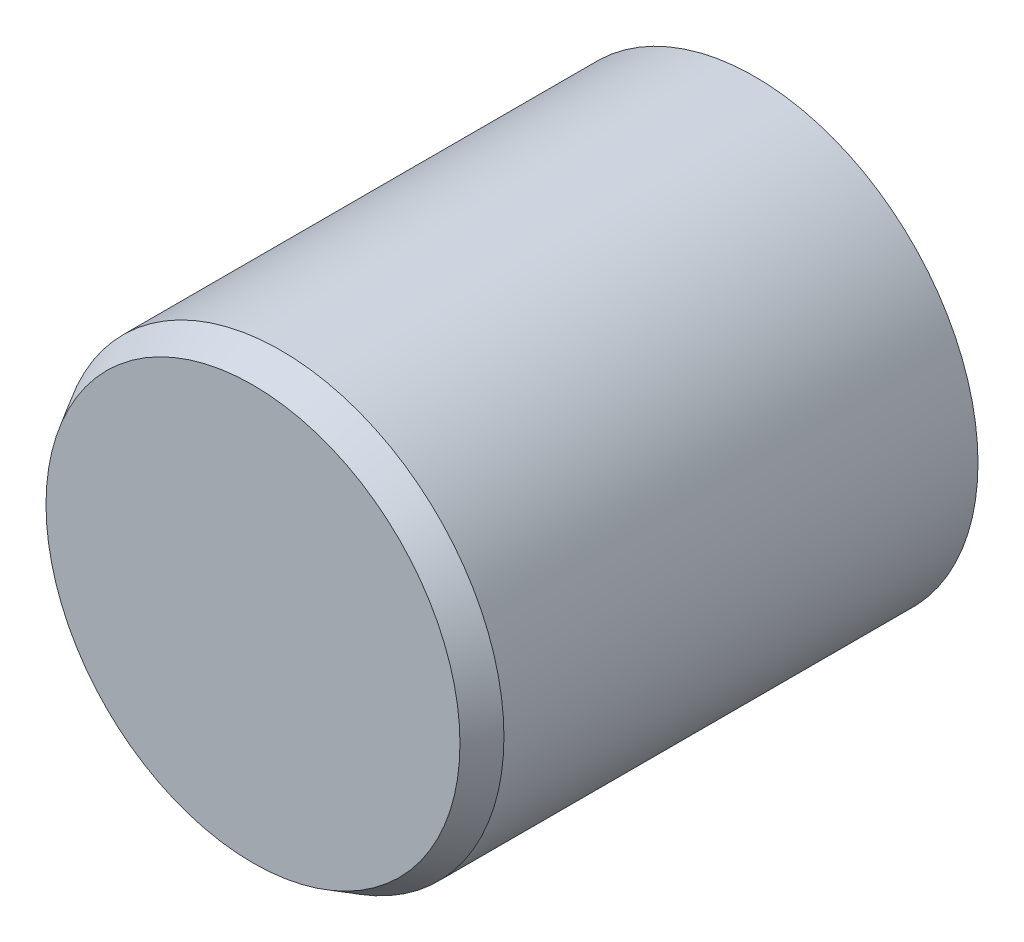
from build123d import *

# Parameters (mm, degrees)
END_CHAMFER_0_5X30DEG_SIZE  = 0.5
END_CHAMFER_0_5X30DEG_SIZE2 = 0.288675135


with BuildPart() as part:
    # Pin Profile Sketch → Pin Body Revolve (revolve)
    with BuildSketch(Plane(origin=(0, 0, 0), x_dir=(0, 0, -1), z_dir=(1, 0, 0)), mode=Mode.PRIVATE) as pin_body_revolve_sk:
        Polygon((0, -1.466666667), (0, -2.966666667), (-9, -2.966666667), (-9, 1.033333333), (-6, 1.033333333), (-6, -1.466666667), align=None)
    revolve(pin_body_revolve_sk.sketch.rotate(Axis((0, 1.033333333, 9), (0, 0, -1)), 270), axis=Axis((0, 1.033333333, 9), (0, 0, -1)))

    # End Chamfer 0.5x30deg
    end_chamfer_0_5x30deg_edges = [part.edges().sort_by_distance(p)[0] for p in [
        (-4, 1.033333333, 9),
    ]]
    end_chamfer_0_5x30deg_side = [part.faces().sort_by_distance(p)[0] for p in [
        (-4, 1.033333333, 4.5),
    ]]
    chamfer(end_chamfer_0_5x30deg_edges, length=END_CHAMFER_0_5X30DEG_SIZE, length2=END_CHAMFER_0_5X30DEG_SIZE2, reference=end_chamfer_0_5x30deg_side[0])


solid = part.part
